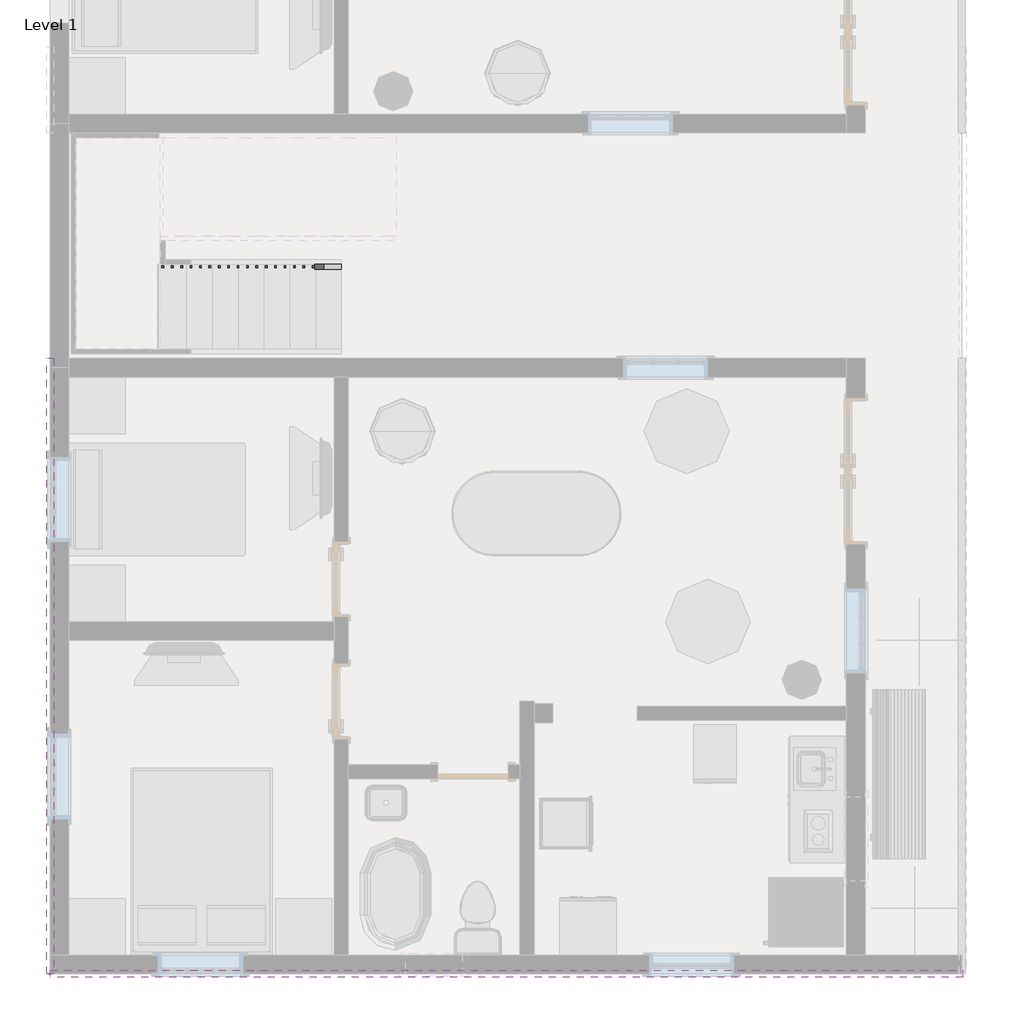
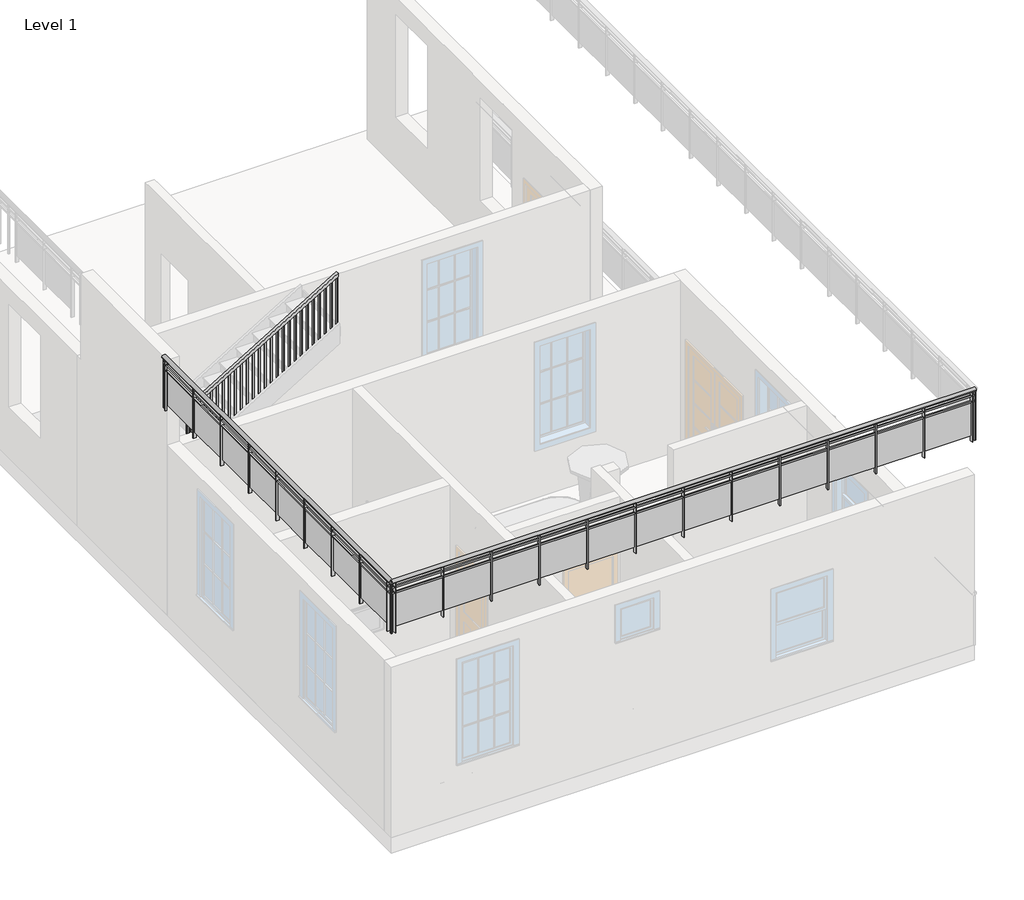
# One storey, part 2 of 4: 3 railings.
"""IFC4 building model written with IfcOpenShell, lengths in millimetres."""

from ifc_helpers import new_model, si_unit, point, frame, origin, place, context, project, spatial, polyline, ellipse_curve, trimmed, outline, extrude, faceted_brep, element, save
from ifc_brep_helpers import plane_surface, extruded_surface, advanced_brep

model = new_model("IFC4")

# Units and contexts
model_context = context("Model", 3, world=origin())
ifc_project = project(units=[si_unit("LENGTHUNIT", "METRE", prefix="MILLI")], contexts=[model_context])

# Site, building, storey
site = spatial("IfcSite", under=ifc_project)
building = spatial("IfcBuilding", under=site)
storey = spatial("IfcBuildingStorey", under=building, Name="Level 1", Elevation=0.0)

# Railings
placement = place(None, origin())
element("IfcRailing", 1, ObjectType="Glass Panel - Bottom Fill", at=placement, inside=storey, context=model_context, shape_type="SolidModel", body=[
    advanced_brep(
    [(-14570.2750862, -617.6379829, 4572.0), (-14570.2750862, -693.8379829, 4572.0), (-4702.3750862, -617.6379829, 4572.0), (-4702.3750862, -693.8379829, 4572.0)],
    [
        (0, 1, ellipse_curve(frame((-14570.2750862, -655.7379829, 4572.0), z_axis=(-1.0, 0.0, 0.0), x_axis=(0.0, -1.0, 0.0)), 38.1, 28.575)),
        (1, 0, ellipse_curve(frame((-14570.2750862, -655.7379829, 4572.0), z_axis=(-1.0, 0.0, 0.0), x_axis=(0.0, -1.0, 0.0)), 38.1, 28.575)),
        (2, 3, ellipse_curve(frame((-4702.3750862, -655.7379829, 4572.0), z_axis=(1.0, 0.0, 0.0), x_axis=(0.0, -1.0, 0.0)), 38.1, 28.575)),
        (3, 2, ellipse_curve(frame((-4702.3750862, -655.7379829, 4572.0), z_axis=(1.0, 0.0, 0.0), x_axis=(0.0, -1.0, 0.0)), 38.1, 28.575)),
        (0, 2),
        (3, 1),
    ],
    [
        plane_surface(frame((-14570.2750862, -655.7379829, 4572.0), z_axis=(-1.0, 0.0, 0.0), x_axis=(0.0, 1.0, 0.0))),
        plane_surface(frame((-4702.3750862, -655.7379829, 4572.0), z_axis=(1.0, 0.0, 0.0), x_axis=(0.0, 1.0, 0.0))),
        extruded_surface(trimmed(ellipse_curve(frame((-4702.3750862, -655.7379829, 4572.0), z_axis=(-1.0, 0.0, 0.0), x_axis=(0.0, -1.0, 0.0)), 38.1, 28.575), [point((-4702.3750862, -617.6379829, 4572.0))], [point((-4702.3750862, -693.8379829, 4572.0))], True, "CARTESIAN"), (-9867.9, 0.0, 0.0), 9867.9),
        extruded_surface(trimmed(ellipse_curve(frame((-4702.3750862, -655.7379829, 4572.0), z_axis=(-1.0, 0.0, 0.0), x_axis=(0.0, -1.0, 0.0)), 38.1, 28.575), [point((-4702.3750862, -693.8379829, 4572.0))], [point((-4702.3750862, -617.6379829, 4572.0))], True, "CARTESIAN"), (-9867.9, 0.0, 0.0), 9867.9),
    ],
    [
        (0, [[1, 2]]),
        (1, [[3, 4]]),
        (2, [[-1, 5, -4, 6]]),
        (3, [[-2, -6, -3, -5]]),
    ],
),
    extrude(outline(polyline([(-14570.2750862, -668.4379829), (-14570.2750862, -643.0379829), (-4702.3750862, -643.0379829), (-4702.3750862, -668.4379829), (-14570.2750862, -668.4379829)])), frame((0.0, 0.0, 4457.7), z_axis=(0.0, 0.0, 1.0), x_axis=(1.0, 0.0, 0.0)), (0.0, 0.0, 1.0), 25.4),
    extrude(outline(polyline([(-14570.2750862, -668.4379829), (-14570.2750862, -643.0379829), (-4702.3750862, -643.0379829), (-4702.3750862, -668.4379829), (-14570.2750862, -668.4379829)])), frame((0.0, 0.0, 4356.1), z_axis=(0.0, 0.0, 1.0), x_axis=(1.0, 0.0, 0.0)), (0.0, 0.0, 1.0), 25.4),
    extrude(outline(polyline([(-4765.8750862, -681.1379829), (-4765.8750862, -630.3379829), (-4753.1750862, -630.3379829), (-4753.1750862, -681.1379829), (-4765.8750862, -681.1379829)])), frame((0.0, 0.0, 3657.6), z_axis=(0.0, 0.0, 1.0), x_axis=(1.0, 0.0, 0.0)), (0.0, 0.0, 1.0), 885.6788223),
    extrude(outline(polyline([(-5572.3250862, -649.2028259), (-4759.5250862, -649.2028259), (-4759.5250862, -655.5528259), (-5572.3250862, -655.5528259), (-5572.3250862, -649.2028259)])), frame((0.0, 0.0, 3759.2), z_axis=(0.0, 0.0, 1.0), x_axis=(1.0, 0.0, 0.0)), (0.0, 0.0, 1.0), 596.9),
    extrude(outline(polyline([(-5578.6750862, -681.1379829), (-5578.6750862, -630.3379829), (-5565.9750862, -630.3379829), (-5565.9750862, -681.1379829), (-5578.6750862, -681.1379829)])), frame((0.0, 0.0, 3657.6), z_axis=(0.0, 0.0, 1.0), x_axis=(1.0, 0.0, 0.0)), (0.0, 0.0, 1.0), 885.6788223),
    extrude(outline(polyline([(-6385.1250862, -649.2028259), (-5572.3250862, -649.2028259), (-5572.3250862, -655.5528259), (-6385.1250862, -655.5528259), (-6385.1250862, -649.2028259)])), frame((0.0, 0.0, 3759.2), z_axis=(0.0, 0.0, 1.0), x_axis=(1.0, 0.0, 0.0)), (0.0, 0.0, 1.0), 596.9),
    extrude(outline(polyline([(-6391.4750862, -681.1379829), (-6391.4750862, -630.3379829), (-6378.7750862, -630.3379829), (-6378.7750862, -681.1379829), (-6391.4750862, -681.1379829)])), frame((0.0, 0.0, 3657.6), z_axis=(0.0, 0.0, 1.0), x_axis=(1.0, 0.0, 0.0)), (0.0, 0.0, 1.0), 885.6788223),
    extrude(outline(polyline([(-7197.9250862, -649.2028259), (-6385.1250862, -649.2028259), (-6385.1250862, -655.5528259), (-7197.9250862, -655.5528259), (-7197.9250862, -649.2028259)])), frame((0.0, 0.0, 3759.2), z_axis=(0.0, 0.0, 1.0), x_axis=(1.0, 0.0, 0.0)), (0.0, 0.0, 1.0), 596.9),
    extrude(outline(polyline([(-7204.2750862, -681.1379829), (-7204.2750862, -630.3379829), (-7191.5750862, -630.3379829), (-7191.5750862, -681.1379829), (-7204.2750862, -681.1379829)])), frame((0.0, 0.0, 3657.6), z_axis=(0.0, 0.0, 1.0), x_axis=(1.0, 0.0, 0.0)), (0.0, 0.0, 1.0), 885.6788223),
    extrude(outline(polyline([(-8010.7250862, -649.2028259), (-7197.9250862, -649.2028259), (-7197.9250862, -655.5528259), (-8010.7250862, -655.5528259), (-8010.7250862, -649.2028259)])), frame((0.0, 0.0, 3759.2), z_axis=(0.0, 0.0, 1.0), x_axis=(1.0, 0.0, 0.0)), (0.0, 0.0, 1.0), 596.9),
    extrude(outline(polyline([(-8017.0750862, -681.1379829), (-8017.0750862, -630.3379829), (-8004.3750862, -630.3379829), (-8004.3750862, -681.1379829), (-8017.0750862, -681.1379829)])), frame((0.0, 0.0, 3657.6), z_axis=(0.0, 0.0, 1.0), x_axis=(1.0, 0.0, 0.0)), (0.0, 0.0, 1.0), 885.6788223),
    extrude(outline(polyline([(-8823.5250862, -649.2028259), (-8010.7250862, -649.2028259), (-8010.7250862, -655.5528259), (-8823.5250862, -655.5528259), (-8823.5250862, -649.2028259)])), frame((0.0, 0.0, 3759.2), z_axis=(0.0, 0.0, 1.0), x_axis=(1.0, 0.0, 0.0)), (0.0, 0.0, 1.0), 596.9),
    extrude(outline(polyline([(-8829.8750862, -681.1379829), (-8829.8750862, -630.3379829), (-8817.1750862, -630.3379829), (-8817.1750862, -681.1379829), (-8829.8750862, -681.1379829)])), frame((0.0, 0.0, 3657.6), z_axis=(0.0, 0.0, 1.0), x_axis=(1.0, 0.0, 0.0)), (0.0, 0.0, 1.0), 885.6788223),
    extrude(outline(polyline([(-9636.3250862, -649.2028259), (-8823.5250862, -649.2028259), (-8823.5250862, -655.5528259), (-9636.3250862, -655.5528259), (-9636.3250862, -649.2028259)])), frame((0.0, 0.0, 3759.2), z_axis=(0.0, 0.0, 1.0), x_axis=(1.0, 0.0, 0.0)), (0.0, 0.0, 1.0), 596.9),
    extrude(outline(polyline([(-9642.6750862, -681.1379829), (-9642.6750862, -630.3379829), (-9629.9750862, -630.3379829), (-9629.9750862, -681.1379829), (-9642.6750862, -681.1379829)])), frame((0.0, 0.0, 3657.6), z_axis=(0.0, 0.0, 1.0), x_axis=(1.0, 0.0, 0.0)), (0.0, 0.0, 1.0), 885.6788223),
    extrude(outline(polyline([(-10449.1250862, -649.2028259), (-9636.3250862, -649.2028259), (-9636.3250862, -655.5528259), (-10449.1250862, -655.5528259), (-10449.1250862, -649.2028259)])), frame((0.0, 0.0, 3759.2), z_axis=(0.0, 0.0, 1.0), x_axis=(1.0, 0.0, 0.0)), (0.0, 0.0, 1.0), 596.9),
    extrude(outline(polyline([(-10455.4750862, -681.1379829), (-10455.4750862, -630.3379829), (-10442.7750862, -630.3379829), (-10442.7750862, -681.1379829), (-10455.4750862, -681.1379829)])), frame((0.0, 0.0, 3657.6), z_axis=(0.0, 0.0, 1.0), x_axis=(1.0, 0.0, 0.0)), (0.0, 0.0, 1.0), 885.6788223),
    extrude(outline(polyline([(-11261.9250862, -649.2028259), (-10449.1250862, -649.2028259), (-10449.1250862, -655.5528259), (-11261.9250862, -655.5528259), (-11261.9250862, -649.2028259)])), frame((0.0, 0.0, 3759.2), z_axis=(0.0, 0.0, 1.0), x_axis=(1.0, 0.0, 0.0)), (0.0, 0.0, 1.0), 596.9),
    extrude(outline(polyline([(-11268.2750862, -681.1379829), (-11268.2750862, -630.3379829), (-11255.5750862, -630.3379829), (-11255.5750862, -681.1379829), (-11268.2750862, -681.1379829)])), frame((0.0, 0.0, 3657.6), z_axis=(0.0, 0.0, 1.0), x_axis=(1.0, 0.0, 0.0)), (0.0, 0.0, 1.0), 885.6788223),
    extrude(outline(polyline([(-12074.7250862, -649.2028259), (-11261.9250862, -649.2028259), (-11261.9250862, -655.5528259), (-12074.7250862, -655.5528259), (-12074.7250862, -649.2028259)])), frame((0.0, 0.0, 3759.2), z_axis=(0.0, 0.0, 1.0), x_axis=(1.0, 0.0, 0.0)), (0.0, 0.0, 1.0), 596.9),
    extrude(outline(polyline([(-12081.0750862, -681.1379829), (-12081.0750862, -630.3379829), (-12068.3750862, -630.3379829), (-12068.3750862, -681.1379829), (-12081.0750862, -681.1379829)])), frame((0.0, 0.0, 3657.6), z_axis=(0.0, 0.0, 1.0), x_axis=(1.0, 0.0, 0.0)), (0.0, 0.0, 1.0), 885.6788223),
    extrude(outline(polyline([(-12887.5250862, -649.2028259), (-12074.7250862, -649.2028259), (-12074.7250862, -655.5528259), (-12887.5250862, -655.5528259), (-12887.5250862, -649.2028259)])), frame((0.0, 0.0, 3759.2), z_axis=(0.0, 0.0, 1.0), x_axis=(1.0, 0.0, 0.0)), (0.0, 0.0, 1.0), 596.9),
    extrude(outline(polyline([(-12893.8750862, -681.1379829), (-12893.8750862, -630.3379829), (-12881.1750862, -630.3379829), (-12881.1750862, -681.1379829), (-12893.8750862, -681.1379829)])), frame((0.0, 0.0, 3657.6), z_axis=(0.0, 0.0, 1.0), x_axis=(1.0, 0.0, 0.0)), (0.0, 0.0, 1.0), 885.6788223),
    extrude(outline(polyline([(-13700.3250862, -649.2028259), (-12887.5250862, -649.2028259), (-12887.5250862, -655.5528259), (-13700.3250862, -655.5528259), (-13700.3250862, -649.2028259)])), frame((0.0, 0.0, 3759.2), z_axis=(0.0, 0.0, 1.0), x_axis=(1.0, 0.0, 0.0)), (0.0, 0.0, 1.0), 596.9),
    extrude(outline(polyline([(-13706.6750862, -681.1379829), (-13706.6750862, -630.3379829), (-13693.9750862, -630.3379829), (-13693.9750862, -681.1379829), (-13706.6750862, -681.1379829)])), frame((0.0, 0.0, 3657.6), z_axis=(0.0, 0.0, 1.0), x_axis=(1.0, 0.0, 0.0)), (0.0, 0.0, 1.0), 885.6788223),
    extrude(outline(polyline([(-14513.1250862, -649.2028259), (-13700.3250862, -649.2028259), (-13700.3250862, -655.5528259), (-14513.1250862, -655.5528259), (-14513.1250862, -649.2028259)])), frame((0.0, 0.0, 3759.2), z_axis=(0.0, 0.0, 1.0), x_axis=(1.0, 0.0, 0.0)), (0.0, 0.0, 1.0), 596.9),
    extrude(outline(polyline([(-14519.4750862, -681.1379829), (-14519.4750862, -630.3379829), (-14506.7750862, -630.3379829), (-14506.7750862, -681.1379829), (-14519.4750862, -681.1379829)])), frame((0.0, 0.0, 3657.6), z_axis=(0.0, 0.0, 1.0), x_axis=(1.0, 0.0, 0.0)), (0.0, 0.0, 1.0), 885.6788223),
    extrude(outline(polyline([(-4715.0750862, -665.2629829), (-4715.0750862, -646.2129829), (-4696.0250862, -646.2129829), (-4696.0250862, -665.2629829), (-4715.0750862, -665.2629829)])), frame((0.0, 0.0, 3657.6), z_axis=(0.0, 0.0, 1.0), x_axis=(1.0, 0.0, 0.0)), (0.0, 0.0, 1.0), 885.6788223),
    extrude(outline(polyline([(-14576.6250862, -665.2629829), (-14576.6250862, -646.2129829), (-14557.5750862, -646.2129829), (-14557.5750862, -665.2629829), (-14576.6250862, -665.2629829)])), frame((0.0, 0.0, 3657.6), z_axis=(0.0, 0.0, 1.0), x_axis=(1.0, 0.0, 0.0)), (0.0, 0.0, 1.0), 885.6788223),
])
element("IfcRailing", 2, ObjectType="Glass Panel - Bottom Fill", at=placement, inside=storey, context=model_context, shape_type="SolidModel", body=[
    advanced_brep(
    [(-14532.1750862, 5999.0620171, 4572.0), (-14608.3750862, 5999.0620171, 4572.0), (-14532.1750862, -655.7379829, 4572.0), (-14608.3750862, -655.7379829, 4572.0)],
    [
        (0, 1, ellipse_curve(frame((-14570.2750862, 5999.0620171, 4572.0), z_axis=(0.0, 1.0, 0.0), x_axis=(-1.0, 0.0, 0.0)), 38.1, 28.575)),
        (1, 0, ellipse_curve(frame((-14570.2750862, 5999.0620171, 4572.0), z_axis=(0.0, 1.0, 0.0), x_axis=(-1.0, 0.0, 0.0)), 38.1, 28.575)),
        (2, 3, ellipse_curve(frame((-14570.2750862, -655.7379829, 4572.0), z_axis=(0.0, -1.0, 0.0), x_axis=(-1.0, 0.0, 0.0)), 38.1, 28.575)),
        (3, 2, ellipse_curve(frame((-14570.2750862, -655.7379829, 4572.0), z_axis=(0.0, -1.0, 0.0), x_axis=(-1.0, 0.0, 0.0)), 38.1, 28.575)),
        (0, 2),
        (3, 1),
    ],
    [
        plane_surface(frame((-14570.2750862, 5999.0620171, 4572.0), z_axis=(0.0, 1.0, 0.0), x_axis=(0.0, 0.0, -1.0))),
        plane_surface(frame((-14570.2750862, -655.7379829, 4572.0), z_axis=(0.0, -1.0, 0.0), x_axis=(0.0, 0.0, -1.0))),
        extruded_surface(trimmed(ellipse_curve(frame((-14570.2750862, -655.7379829, 4572.0), z_axis=(0.0, 1.0, 0.0), x_axis=(-1.0, 0.0, 0.0)), 38.1, 28.575), [point((-14532.1750862, -655.7379829, 4572.0))], [point((-14608.3750862, -655.7379829, 4572.0))], True, "CARTESIAN"), (0.0, 6654.8, 0.0), 6654.8),
        extruded_surface(trimmed(ellipse_curve(frame((-14570.2750862, -655.7379829, 4572.0), z_axis=(0.0, 1.0, 0.0), x_axis=(-1.0, 0.0, 0.0)), 38.1, 28.575), [point((-14608.3750862, -655.7379829, 4572.0))], [point((-14532.1750862, -655.7379829, 4572.0))], True, "CARTESIAN"), (0.0, 6654.8, 0.0), 6654.8),
    ],
    [
        (0, [[1, 2]]),
        (1, [[3, 4]]),
        (2, [[-1, 5, -4, 6]]),
        (3, [[-2, -6, -3, -5]]),
    ],
),
    extrude(outline(polyline([(-14582.9750862, 5999.0620171), (-14557.5750862, 5999.0620171), (-14557.5750862, -655.7379829), (-14582.9750862, -655.7379829), (-14582.9750862, 5999.0620171)])), frame((0.0, 0.0, 4457.7), z_axis=(0.0, 0.0, 1.0), x_axis=(1.0, 0.0, 0.0)), (0.0, 0.0, 1.0), 25.4),
    extrude(outline(polyline([(-14582.9750862, 5999.0620171), (-14557.5750862, 5999.0620171), (-14557.5750862, -655.7379829), (-14582.9750862, -655.7379829), (-14582.9750862, 5999.0620171)])), frame((0.0, 0.0, 4356.1), z_axis=(0.0, 0.0, 1.0), x_axis=(1.0, 0.0, 0.0)), (0.0, 0.0, 1.0), 25.4),
    extrude(outline(polyline([(-14595.6750862, -573.1879829), (-14544.8750862, -573.1879829), (-14544.8750862, -585.8879829), (-14595.6750862, -585.8879829), (-14595.6750862, -573.1879829)])), frame((0.0, 0.0, 3657.6), z_axis=(0.0, 0.0, 1.0), x_axis=(1.0, 0.0, 0.0)), (0.0, 0.0, 1.0), 885.6788223),
    extrude(outline(polyline([(-14563.7399292, 233.2620171), (-14563.7399292, -579.5379829), (-14570.0899292, -579.5379829), (-14570.0899292, 233.2620171), (-14563.7399292, 233.2620171)])), frame((0.0, 0.0, 3759.2), z_axis=(0.0, 0.0, 1.0), x_axis=(1.0, 0.0, 0.0)), (0.0, 0.0, 1.0), 596.9),
    extrude(outline(polyline([(-14595.6750862, 239.6120171), (-14544.8750862, 239.6120171), (-14544.8750862, 226.9120171), (-14595.6750862, 226.9120171), (-14595.6750862, 239.6120171)])), frame((0.0, 0.0, 3657.6), z_axis=(0.0, 0.0, 1.0), x_axis=(1.0, 0.0, 0.0)), (0.0, 0.0, 1.0), 885.6788223),
    extrude(outline(polyline([(-14563.7399292, 1046.0620171), (-14563.7399292, 233.2620171), (-14570.0899292, 233.2620171), (-14570.0899292, 1046.0620171), (-14563.7399292, 1046.0620171)])), frame((0.0, 0.0, 3759.2), z_axis=(0.0, 0.0, 1.0), x_axis=(1.0, 0.0, 0.0)), (0.0, 0.0, 1.0), 596.9),
    extrude(outline(polyline([(-14595.6750862, 1052.4120171), (-14544.8750862, 1052.4120171), (-14544.8750862, 1039.7120171), (-14595.6750862, 1039.7120171), (-14595.6750862, 1052.4120171)])), frame((0.0, 0.0, 3657.6), z_axis=(0.0, 0.0, 1.0), x_axis=(1.0, 0.0, 0.0)), (0.0, 0.0, 1.0), 885.6788223),
    extrude(outline(polyline([(-14563.7399292, 1858.8620171), (-14563.7399292, 1046.0620171), (-14570.0899292, 1046.0620171), (-14570.0899292, 1858.8620171), (-14563.7399292, 1858.8620171)])), frame((0.0, 0.0, 3759.2), z_axis=(0.0, 0.0, 1.0), x_axis=(1.0, 0.0, 0.0)), (0.0, 0.0, 1.0), 596.9),
    extrude(outline(polyline([(-14595.6750862, 1865.2120171), (-14544.8750862, 1865.2120171), (-14544.8750862, 1852.5120171), (-14595.6750862, 1852.5120171), (-14595.6750862, 1865.2120171)])), frame((0.0, 0.0, 3657.6), z_axis=(0.0, 0.0, 1.0), x_axis=(1.0, 0.0, 0.0)), (0.0, 0.0, 1.0), 885.6788223),
    extrude(outline(polyline([(-14563.7399292, 2671.6620171), (-14563.7399292, 1858.8620171), (-14570.0899292, 1858.8620171), (-14570.0899292, 2671.6620171), (-14563.7399292, 2671.6620171)])), frame((0.0, 0.0, 3759.2), z_axis=(0.0, 0.0, 1.0), x_axis=(1.0, 0.0, 0.0)), (0.0, 0.0, 1.0), 596.9),
    extrude(outline(polyline([(-14595.6750862, 2678.0120171), (-14544.8750862, 2678.0120171), (-14544.8750862, 2665.3120171), (-14595.6750862, 2665.3120171), (-14595.6750862, 2678.0120171)])), frame((0.0, 0.0, 3657.6), z_axis=(0.0, 0.0, 1.0), x_axis=(1.0, 0.0, 0.0)), (0.0, 0.0, 1.0), 885.6788223),
    extrude(outline(polyline([(-14563.7399292, 3484.4620171), (-14563.7399292, 2671.6620171), (-14570.0899292, 2671.6620171), (-14570.0899292, 3484.4620171), (-14563.7399292, 3484.4620171)])), frame((0.0, 0.0, 3759.2), z_axis=(0.0, 0.0, 1.0), x_axis=(1.0, 0.0, 0.0)), (0.0, 0.0, 1.0), 596.9),
    extrude(outline(polyline([(-14595.6750862, 3490.8120171), (-14544.8750862, 3490.8120171), (-14544.8750862, 3478.1120171), (-14595.6750862, 3478.1120171), (-14595.6750862, 3490.8120171)])), frame((0.0, 0.0, 3657.6), z_axis=(0.0, 0.0, 1.0), x_axis=(1.0, 0.0, 0.0)), (0.0, 0.0, 1.0), 885.6788223),
    extrude(outline(polyline([(-14563.7399292, 4297.2620171), (-14563.7399292, 3484.4620171), (-14570.0899292, 3484.4620171), (-14570.0899292, 4297.2620171), (-14563.7399292, 4297.2620171)])), frame((0.0, 0.0, 3759.2), z_axis=(0.0, 0.0, 1.0), x_axis=(1.0, 0.0, 0.0)), (0.0, 0.0, 1.0), 596.9),
    extrude(outline(polyline([(-14595.6750862, 4303.6120171), (-14544.8750862, 4303.6120171), (-14544.8750862, 4290.9120171), (-14595.6750862, 4290.9120171), (-14595.6750862, 4303.6120171)])), frame((0.0, 0.0, 3657.6), z_axis=(0.0, 0.0, 1.0), x_axis=(1.0, 0.0, 0.0)), (0.0, 0.0, 1.0), 885.6788223),
    extrude(outline(polyline([(-14563.7399292, 5110.0620171), (-14563.7399292, 4297.2620171), (-14570.0899292, 4297.2620171), (-14570.0899292, 5110.0620171), (-14563.7399292, 5110.0620171)])), frame((0.0, 0.0, 3759.2), z_axis=(0.0, 0.0, 1.0), x_axis=(1.0, 0.0, 0.0)), (0.0, 0.0, 1.0), 596.9),
    extrude(outline(polyline([(-14595.6750862, 5116.4120171), (-14544.8750862, 5116.4120171), (-14544.8750862, 5103.7120171), (-14595.6750862, 5103.7120171), (-14595.6750862, 5116.4120171)])), frame((0.0, 0.0, 3657.6), z_axis=(0.0, 0.0, 1.0), x_axis=(1.0, 0.0, 0.0)), (0.0, 0.0, 1.0), 885.6788223),
    extrude(outline(polyline([(-14563.7399292, 5922.8620171), (-14563.7399292, 5110.0620171), (-14570.0899292, 5110.0620171), (-14570.0899292, 5922.8620171), (-14563.7399292, 5922.8620171)])), frame((0.0, 0.0, 3759.2), z_axis=(0.0, 0.0, 1.0), x_axis=(1.0, 0.0, 0.0)), (0.0, 0.0, 1.0), 596.9),
    extrude(outline(polyline([(-14595.6750862, 5929.2120171), (-14544.8750862, 5929.2120171), (-14544.8750862, 5916.5120171), (-14595.6750862, 5916.5120171), (-14595.6750862, 5929.2120171)])), frame((0.0, 0.0, 3657.6), z_axis=(0.0, 0.0, 1.0), x_axis=(1.0, 0.0, 0.0)), (0.0, 0.0, 1.0), 885.6788223),
    extrude(outline(polyline([(-14579.8000862, -643.0379829), (-14560.7500862, -643.0379829), (-14560.7500862, -662.0879829), (-14579.8000862, -662.0879829), (-14579.8000862, -643.0379829)])), frame((0.0, 0.0, 3657.6), z_axis=(0.0, 0.0, 1.0), x_axis=(1.0, 0.0, 0.0)), (0.0, 0.0, 1.0), 885.6788223),
    extrude(outline(polyline([(-14579.8000862, 6005.4120171), (-14560.7500862, 6005.4120171), (-14560.7500862, 5986.3620171), (-14579.8000862, 5986.3620171), (-14579.8000862, 6005.4120171)])), frame((0.0, 0.0, 3657.6), z_axis=(0.0, 0.0, 1.0), x_axis=(1.0, 0.0, 0.0)), (0.0, 0.0, 1.0), 885.6788223),
])
element("IfcRailing", 3, ObjectType="Handrail - Rectangular", at=placement, inside=storey, context=model_context, shape_type="SolidModel", body=[
    faceted_brep([(-11420.6750862, 6964.2620171, 1083.7333333), (-11420.6750862, 6964.2620171, 1024.3318731), (-11420.6750862, 7015.0620171, 1024.3318731), (-11420.6750862, 7015.0620171, 1083.7333333), (-13300.2750862, 6964.2620171, 2222.8848485), (-13351.0750862, 6964.2620171, 2194.271267), (-13351.0750862, 7015.0620171, 2194.271267), (-13300.2750862, 7015.0620171, 2222.8848485), (-13300.2750862, 6964.2620171, 2269.0666667), (-13351.0750862, 6964.2620171, 2218.2666667), (-13351.0750862, 7015.0620171, 2218.2666667), (-13300.2750862, 7015.0620171, 2269.0666667), (-13427.2750862, 6964.2620171, 2269.0666667), (-13427.2750862, 6964.2620171, 2218.2666667), (-13376.4750862, 7015.0620171, 2218.2666667), (-13376.4750862, 7015.0620171, 2269.0666667), (-13427.2750862, 7091.2620171, 2269.0666667), (-13427.2750862, 7091.2620171, 2218.2666667), (-13376.4750862, 7091.2620171, 2218.2666667), (-13376.4750862, 7091.2620171, 2269.0666667), (-13427.2750862, 7243.6620171, 2269.0666667), (-13427.2750862, 7294.4620171, 2218.2666667), (-13376.4750862, 7294.4620171, 2218.2666667), (-13376.4750862, 7243.6620171, 2269.0666667), (-13427.2750862, 7243.6620171, 2484.5818182), (-13427.2750862, 7294.4620171, 2433.7818182), (-13376.4750862, 7294.4620171, 2433.7818182), (-13376.4750862, 7243.6620171, 2484.5818182), (-13427.2750862, 7370.6620171, 2484.5818182), (-13427.2750862, 7370.6620171, 2433.7818182), (-13376.4750862, 7319.8620171, 2433.7818182), (-13376.4750862, 7319.8620171, 2484.5818182), (-13300.2750862, 7370.6620171, 2484.5818182), (-13286.0826767, 7370.6620171, 2433.7818182), (-13286.0826767, 7319.8620171, 2433.7818182), (-13300.2750862, 7319.8620171, 2484.5818182), (-10861.8750862, 7370.6620171, 3962.4), (-10861.8750862, 7319.8620171, 3962.4), (-10861.8750862, 7319.8620171, 3902.9985397), (-10861.8750862, 7370.6620171, 3902.9985397)], [[[0, 1, 2, 3]], [[1, 0, 4, 5]], [[2, 1, 5, 6]], [[3, 2, 6, 7]], [[0, 3, 7, 4]], [[5, 4, 8, 9]], [[6, 5, 9, 10]], [[7, 6, 10, 11]], [[4, 7, 11, 8]], [[9, 8, 12, 13]], [[10, 9, 13, 14]], [[11, 10, 14, 15]], [[8, 11, 15, 12]], [[13, 12, 16, 17]], [[14, 13, 17, 18]], [[15, 14, 18, 19]], [[12, 15, 19, 16]], [[17, 16, 20, 21]], [[18, 17, 21, 22]], [[19, 18, 22, 23]], [[16, 19, 23, 20]], [[21, 20, 24, 25]], [[22, 21, 25, 26]], [[23, 22, 26, 27]], [[20, 23, 27, 24]], [[25, 24, 28, 29]], [[26, 25, 29, 30]], [[27, 26, 30, 31]], [[24, 27, 31, 28]], [[29, 28, 32, 33]], [[30, 29, 33, 34]], [[31, 30, 34, 35]], [[28, 31, 35, 32]], [[36, 37, 38, 39]], [[33, 32, 36, 39]], [[34, 33, 39, 38]], [[35, 34, 38, 37]], [[32, 35, 37, 36]]]),
    extrude(outline(polyline([(3847.1955094, -10953.9500862), (3835.6500549, -10973.0000862), (2878.6666667, -10973.0000862), (2878.6666667, -10953.9500862), (3847.1955094, -10953.9500862)])), frame((0.0, 7335.7370171, 0.0), z_axis=(0.0, 1.0, 0.0), x_axis=(0.0, 0.0, 1.0)), (0.0, 0.0, 1.0), 19.05),
    extrude(outline(polyline([(3785.6197519, -11055.5500862), (3774.0742973, -11074.6000862), (2878.6666667, -11074.6000862), (2878.6666667, -11055.5500862), (3785.6197519, -11055.5500862)])), frame((0.0, 7335.7370171, 0.0), z_axis=(0.0, 1.0, 0.0), x_axis=(0.0, 0.0, 1.0)), (0.0, 0.0, 1.0), 19.05),
    extrude(outline(polyline([(3724.0439943, -11157.1500862), (3712.4985397, -11176.2000862), (2709.3333333, -11176.2000862), (2709.3333333, -11157.1500862), (3724.0439943, -11157.1500862)])), frame((0.0, 7335.7370171, 0.0), z_axis=(0.0, 1.0, 0.0), x_axis=(0.0, 0.0, 1.0)), (0.0, 0.0, 1.0), 19.05),
    extrude(outline(polyline([(3662.4682367, -11258.7500862), (3650.9227822, -11277.8000862), (2709.3333333, -11277.8000862), (2709.3333333, -11258.7500862), (3662.4682367, -11258.7500862)])), frame((0.0, 7335.7370171, 0.0), z_axis=(0.0, 1.0, 0.0), x_axis=(0.0, 0.0, 1.0)), (0.0, 0.0, 1.0), 19.05),
    extrude(outline(polyline([(3600.8924791, -11360.3500862), (3589.3470246, -11379.4000862), (2709.3333333, -11379.4000862), (2709.3333333, -11360.3500862), (3600.8924791, -11360.3500862)])), frame((0.0, 7335.7370171, 0.0), z_axis=(0.0, 1.0, 0.0), x_axis=(0.0, 0.0, 1.0)), (0.0, 0.0, 1.0), 19.05),
    extrude(outline(polyline([(3539.3167216, -11461.9500862), (3527.771267, -11481.0000862), (2540.0, -11481.0000862), (2540.0, -11461.9500862), (3539.3167216, -11461.9500862)])), frame((0.0, 7335.7370171, 0.0), z_axis=(0.0, 1.0, 0.0), x_axis=(0.0, 0.0, 1.0)), (0.0, 0.0, 1.0), 19.05),
    extrude(outline(polyline([(3477.740964, -11563.5500862), (3466.1955094, -11582.6000862), (2540.0, -11582.6000862), (2540.0, -11563.5500862), (3477.740964, -11563.5500862)])), frame((0.0, 7335.7370171, 0.0), z_axis=(0.0, 1.0, 0.0), x_axis=(0.0, 0.0, 1.0)), (0.0, 0.0, 1.0), 19.05),
    extrude(outline(polyline([(3416.1652064, -11665.1500862), (3404.6197519, -11684.2000862), (2540.0, -11684.2000862), (2540.0, -11665.1500862), (3416.1652064, -11665.1500862)])), frame((0.0, 7335.7370171, 0.0), z_axis=(0.0, 1.0, 0.0), x_axis=(0.0, 0.0, 1.0)), (0.0, 0.0, 1.0), 19.05),
    extrude(outline(polyline([(3354.5894488, -11766.7500862), (3343.0439943, -11785.8000862), (2370.6666667, -11785.8000862), (2370.6666667, -11766.7500862), (3354.5894488, -11766.7500862)])), frame((0.0, 7335.7370171, 0.0), z_axis=(0.0, 1.0, 0.0), x_axis=(0.0, 0.0, 1.0)), (0.0, 0.0, 1.0), 19.05),
    extrude(outline(polyline([(3293.0136913, -11868.3500862), (3281.4682367, -11887.4000862), (2370.6666667, -11887.4000862), (2370.6666667, -11868.3500862), (3293.0136913, -11868.3500862)])), frame((0.0, 7335.7370171, 0.0), z_axis=(0.0, 1.0, 0.0), x_axis=(0.0, 0.0, 1.0)), (0.0, 0.0, 1.0), 19.05),
    extrude(outline(polyline([(3231.4379337, -11969.9500862), (3219.8924791, -11989.0000862), (2370.6666667, -11989.0000862), (2370.6666667, -11969.9500862), (3231.4379337, -11969.9500862)])), frame((0.0, 7335.7370171, 0.0), z_axis=(0.0, 1.0, 0.0), x_axis=(0.0, 0.0, 1.0)), (0.0, 0.0, 1.0), 19.05),
    extrude(outline(polyline([(3169.8621761, -12071.5500862), (3158.3167216, -12090.6000862), (2201.3333333, -12090.6000862), (2201.3333333, -12071.5500862), (3169.8621761, -12071.5500862)])), frame((0.0, 7335.7370171, 0.0), z_axis=(0.0, 1.0, 0.0), x_axis=(0.0, 0.0, 1.0)), (0.0, 0.0, 1.0), 19.05),
    extrude(outline(polyline([(3108.2864185, -12173.1500862), (3096.740964, -12192.2000862), (2201.3333333, -12192.2000862), (2201.3333333, -12173.1500862), (3108.2864185, -12173.1500862)])), frame((0.0, 7335.7370171, 0.0), z_axis=(0.0, 1.0, 0.0), x_axis=(0.0, 0.0, 1.0)), (0.0, 0.0, 1.0), 19.05),
    extrude(outline(polyline([(3046.710661, -12274.7500862), (3035.1652064, -12293.8000862), (2032.0, -12293.8000862), (2032.0, -12274.7500862), (3046.710661, -12274.7500862)])), frame((0.0, 7335.7370171, 0.0), z_axis=(0.0, 1.0, 0.0), x_axis=(0.0, 0.0, 1.0)), (0.0, 0.0, 1.0), 19.05),
    extrude(outline(polyline([(2985.1349034, -12376.3500862), (2973.5894488, -12395.4000862), (2032.0, -12395.4000862), (2032.0, -12376.3500862), (2985.1349034, -12376.3500862)])), frame((0.0, 7335.7370171, 0.0), z_axis=(0.0, 1.0, 0.0), x_axis=(0.0, 0.0, 1.0)), (0.0, 0.0, 1.0), 19.05),
    extrude(outline(polyline([(2923.5591458, -12477.9500862), (2912.0136913, -12497.0000862), (2032.0, -12497.0000862), (2032.0, -12477.9500862), (2923.5591458, -12477.9500862)])), frame((0.0, 7335.7370171, 0.0), z_axis=(0.0, 1.0, 0.0), x_axis=(0.0, 0.0, 1.0)), (0.0, 0.0, 1.0), 19.05),
    extrude(outline(polyline([(2861.9833882, -12579.5500862), (2850.4379337, -12598.6000862), (1862.6666667, -12598.6000862), (1862.6666667, -12579.5500862), (2861.9833882, -12579.5500862)])), frame((0.0, 7335.7370171, 0.0), z_axis=(0.0, 1.0, 0.0), x_axis=(0.0, 0.0, 1.0)), (0.0, 0.0, 1.0), 19.05),
    extrude(outline(polyline([(2800.4076307, -12681.1500862), (2788.8621761, -12700.2000862), (1862.6666667, -12700.2000862), (1862.6666667, -12681.1500862), (2800.4076307, -12681.1500862)])), frame((0.0, 7335.7370171, 0.0), z_axis=(0.0, 1.0, 0.0), x_axis=(0.0, 0.0, 1.0)), (0.0, 0.0, 1.0), 19.05),
    extrude(outline(polyline([(2738.8318731, -12782.7500862), (2727.2864185, -12801.8000862), (1862.6666667, -12801.8000862), (1862.6666667, -12782.7500862), (2738.8318731, -12782.7500862)])), frame((0.0, 7335.7370171, 0.0), z_axis=(0.0, 1.0, 0.0), x_axis=(0.0, 0.0, 1.0)), (0.0, 0.0, 1.0), 19.05),
    extrude(outline(polyline([(2677.2561155, -12884.3500862), (2665.710661, -12903.4000862), (1693.3333333, -12903.4000862), (1693.3333333, -12884.3500862), (2677.2561155, -12884.3500862)])), frame((0.0, 7335.7370171, 0.0), z_axis=(0.0, 1.0, 0.0), x_axis=(0.0, 0.0, 1.0)), (0.0, 0.0, 1.0), 19.05),
    extrude(outline(polyline([(2615.6803579, -12985.9500862), (2604.1349034, -13005.0000862), (1693.3333333, -13005.0000862), (1693.3333333, -12985.9500862), (2615.6803579, -12985.9500862)])), frame((0.0, 7335.7370171, 0.0), z_axis=(0.0, 1.0, 0.0), x_axis=(0.0, 0.0, 1.0)), (0.0, 0.0, 1.0), 19.05),
    extrude(outline(polyline([(2554.1046004, -13087.5500862), (2542.5591458, -13106.6000862), (1693.3333333, -13106.6000862), (1693.3333333, -13087.5500862), (2554.1046004, -13087.5500862)])), frame((0.0, 7335.7370171, 0.0), z_axis=(0.0, 1.0, 0.0), x_axis=(0.0, 0.0, 1.0)), (0.0, 0.0, 1.0), 19.05),
    extrude(outline(polyline([(2492.5288428, -13189.1500862), (2480.9833882, -13208.2000862), (1524.0, -13208.2000862), (1524.0, -13189.1500862), (2492.5288428, -13189.1500862)])), frame((0.0, 7335.7370171, 0.0), z_axis=(0.0, 1.0, 0.0), x_axis=(0.0, 0.0, 1.0)), (0.0, 0.0, 1.0), 19.05),
    extrude(outline(polyline([(-13309.8000862, 7335.7370171), (-13309.8000862, 7354.7870171), (-13290.7500862, 7354.7870171), (-13290.7500862, 7335.7370171), (-13309.8000862, 7335.7370171)])), frame((0.0, 0.0, 1524.0), z_axis=(0.0, 0.0, 1.0), x_axis=(1.0, 0.0, 0.0)), (0.0, 0.0, 1.0), 909.7818182),
    extrude(outline(polyline([(-13392.3500862, 7284.9370171), (-13411.4000862, 7284.9370171), (-13411.4000862, 7303.9870171), (-13392.3500862, 7303.9870171), (-13392.3500862, 7284.9370171)])), frame((0.0, 0.0, 1354.6666667), z_axis=(0.0, 0.0, 1.0), x_axis=(1.0, 0.0, 0.0)), (0.0, 0.0, 1.0), 863.6),
    extrude(outline(polyline([(-13392.3500862, 7183.3370171), (-13411.4000862, 7183.3370171), (-13411.4000862, 7202.3870171), (-13392.3500862, 7202.3870171), (-13392.3500862, 7183.3370171)])), frame((0.0, 0.0, 1354.6666667), z_axis=(0.0, 0.0, 1.0), x_axis=(1.0, 0.0, 0.0)), (0.0, 0.0, 1.0), 863.6),
    extrude(outline(polyline([(-13392.3500862, 7081.7370171), (-13411.4000862, 7081.7370171), (-13411.4000862, 7100.7870171), (-13392.3500862, 7100.7870171), (-13392.3500862, 7081.7370171)])), frame((0.0, 0.0, 1354.6666667), z_axis=(0.0, 0.0, 1.0), x_axis=(1.0, 0.0, 0.0)), (0.0, 0.0, 1.0), 863.6),
    extrude(outline(polyline([(2188.4985397, -13341.5500862), (2200.0439943, -13360.6000862), (1185.3333333, -13360.6000862), (1185.3333333, -13341.5500862), (2188.4985397, -13341.5500862)])), frame((0.0, 6980.1370171, 0.0), z_axis=(0.0, 1.0, 0.0), x_axis=(0.0, 0.0, 1.0)), (0.0, 0.0, 1.0), 19.05),
    extrude(outline(polyline([(2126.9227822, -13239.9500862), (2138.4682367, -13259.0000862), (1185.3333333, -13259.0000862), (1185.3333333, -13239.9500862), (2126.9227822, -13239.9500862)])), frame((0.0, 6980.1370171, 0.0), z_axis=(0.0, 1.0, 0.0), x_axis=(0.0, 0.0, 1.0)), (0.0, 0.0, 1.0), 19.05),
    extrude(outline(polyline([(2065.3470246, -13138.3500862), (2076.8924791, -13157.4000862), (1185.3333333, -13157.4000862), (1185.3333333, -13138.3500862), (2065.3470246, -13138.3500862)])), frame((0.0, 6980.1370171, 0.0), z_axis=(0.0, 1.0, 0.0), x_axis=(0.0, 0.0, 1.0)), (0.0, 0.0, 1.0), 19.05),
    extrude(outline(polyline([(2003.771267, -13036.7500862), (2015.3167216, -13055.8000862), (1016.0, -13055.8000862), (1016.0, -13036.7500862), (2003.771267, -13036.7500862)])), frame((0.0, 6980.1370171, 0.0), z_axis=(0.0, 1.0, 0.0), x_axis=(0.0, 0.0, 1.0)), (0.0, 0.0, 1.0), 19.05),
    extrude(outline(polyline([(1942.1955094, -12935.1500862), (1953.740964, -12954.2000862), (1016.0, -12954.2000862), (1016.0, -12935.1500862), (1942.1955094, -12935.1500862)])), frame((0.0, 6980.1370171, 0.0), z_axis=(0.0, 1.0, 0.0), x_axis=(0.0, 0.0, 1.0)), (0.0, 0.0, 1.0), 19.05),
    extrude(outline(polyline([(1880.6197519, -12833.5500862), (1892.1652064, -12852.6000862), (1016.0, -12852.6000862), (1016.0, -12833.5500862), (1880.6197519, -12833.5500862)])), frame((0.0, 6980.1370171, 0.0), z_axis=(0.0, 1.0, 0.0), x_axis=(0.0, 0.0, 1.0)), (0.0, 0.0, 1.0), 19.05),
    extrude(outline(polyline([(1819.0439943, -12731.9500862), (1830.5894488, -12751.0000862), (846.6666667, -12751.0000862), (846.6666667, -12731.9500862), (1819.0439943, -12731.9500862)])), frame((0.0, 6980.1370171, 0.0), z_axis=(0.0, 1.0, 0.0), x_axis=(0.0, 0.0, 1.0)), (0.0, 0.0, 1.0), 19.05),
    extrude(outline(polyline([(1757.4682367, -12630.3500862), (1769.0136913, -12649.4000862), (846.6666667, -12649.4000862), (846.6666667, -12630.3500862), (1757.4682367, -12630.3500862)])), frame((0.0, 6980.1370171, 0.0), z_axis=(0.0, 1.0, 0.0), x_axis=(0.0, 0.0, 1.0)), (0.0, 0.0, 1.0), 19.05),
    extrude(outline(polyline([(1695.8924791, -12528.7500862), (1707.4379337, -12547.8000862), (846.6666667, -12547.8000862), (846.6666667, -12528.7500862), (1695.8924791, -12528.7500862)])), frame((0.0, 6980.1370171, 0.0), z_axis=(0.0, 1.0, 0.0), x_axis=(0.0, 0.0, 1.0)), (0.0, 0.0, 1.0), 19.05),
    extrude(outline(polyline([(1634.3167216, -12427.1500862), (1645.8621761, -12446.2000862), (677.3333333, -12446.2000862), (677.3333333, -12427.1500862), (1634.3167216, -12427.1500862)])), frame((0.0, 6980.1370171, 0.0), z_axis=(0.0, 1.0, 0.0), x_axis=(0.0, 0.0, 1.0)), (0.0, 0.0, 1.0), 19.05),
    extrude(outline(polyline([(1572.740964, -12325.5500862), (1584.2864185, -12344.6000862), (677.3333333, -12344.6000862), (677.3333333, -12325.5500862), (1572.740964, -12325.5500862)])), frame((0.0, 6980.1370171, 0.0), z_axis=(0.0, 1.0, 0.0), x_axis=(0.0, 0.0, 1.0)), (0.0, 0.0, 1.0), 19.05),
    extrude(outline(polyline([(1511.1652064, -12223.9500862), (1522.710661, -12243.0000862), (508.0, -12243.0000862), (508.0, -12223.9500862), (1511.1652064, -12223.9500862)])), frame((0.0, 6980.1370171, 0.0), z_axis=(0.0, 1.0, 0.0), x_axis=(0.0, 0.0, 1.0)), (0.0, 0.0, 1.0), 19.05),
    extrude(outline(polyline([(1449.5894488, -12122.3500862), (1461.1349034, -12141.4000862), (508.0, -12141.4000862), (508.0, -12122.3500862), (1449.5894488, -12122.3500862)])), frame((0.0, 6980.1370171, 0.0), z_axis=(0.0, 1.0, 0.0), x_axis=(0.0, 0.0, 1.0)), (0.0, 0.0, 1.0), 19.05),
    extrude(outline(polyline([(1388.0136913, -12020.7500862), (1399.5591458, -12039.8000862), (508.0, -12039.8000862), (508.0, -12020.7500862), (1388.0136913, -12020.7500862)])), frame((0.0, 6980.1370171, 0.0), z_axis=(0.0, 1.0, 0.0), x_axis=(0.0, 0.0, 1.0)), (0.0, 0.0, 1.0), 19.05),
    extrude(outline(polyline([(1326.4379337, -11919.1500862), (1337.9833882, -11938.2000862), (338.6666667, -11938.2000862), (338.6666667, -11919.1500862), (1326.4379337, -11919.1500862)])), frame((0.0, 6980.1370171, 0.0), z_axis=(0.0, 1.0, 0.0), x_axis=(0.0, 0.0, 1.0)), (0.0, 0.0, 1.0), 19.05),
    extrude(outline(polyline([(1264.8621761, -11817.5500862), (1276.4076307, -11836.6000862), (338.6666667, -11836.6000862), (338.6666667, -11817.5500862), (1264.8621761, -11817.5500862)])), frame((0.0, 6980.1370171, 0.0), z_axis=(0.0, 1.0, 0.0), x_axis=(0.0, 0.0, 1.0)), (0.0, 0.0, 1.0), 19.05),
    extrude(outline(polyline([(1203.2864185, -11715.9500862), (1214.8318731, -11735.0000862), (338.6666667, -11735.0000862), (338.6666667, -11715.9500862), (1203.2864185, -11715.9500862)])), frame((0.0, 6980.1370171, 0.0), z_axis=(0.0, 1.0, 0.0), x_axis=(0.0, 0.0, 1.0)), (0.0, 0.0, 1.0), 19.05),
    extrude(outline(polyline([(1141.710661, -11614.3500862), (1153.2561155, -11633.4000862), (169.3333333, -11633.4000862), (169.3333333, -11614.3500862), (1141.710661, -11614.3500862)])), frame((0.0, 6980.1370171, 0.0), z_axis=(0.0, 1.0, 0.0), x_axis=(0.0, 0.0, 1.0)), (0.0, 0.0, 1.0), 19.05),
    extrude(outline(polyline([(1080.1349034, -11512.7500862), (1091.6803579, -11531.8000862), (169.3333333, -11531.8000862), (169.3333333, -11512.7500862), (1080.1349034, -11512.7500862)])), frame((0.0, 6980.1370171, 0.0), z_axis=(0.0, 1.0, 0.0), x_axis=(0.0, 0.0, 1.0)), (0.0, 0.0, 1.0), 19.05),
    extrude(outline(polyline([(-13411.4000862, 7335.7370171), (-13411.4000862, 7354.7870171), (-13392.3500862, 7354.7870171), (-13392.3500862, 7335.7370171), (-13411.4000862, 7335.7370171)])), frame((0.0, 0.0, 1354.6666667), z_axis=(0.0, 0.0, 1.0), x_axis=(1.0, 0.0, 0.0)), (0.0, 0.0, 1.0), 1079.1151515),
    extrude(outline(polyline([(-13392.3500862, 6999.1870171), (-13392.3500862, 6980.1370171), (-13411.4000862, 6980.1370171), (-13411.4000862, 6999.1870171), (-13392.3500862, 6999.1870171)])), frame((0.0, 0.0, 1354.6666667), z_axis=(0.0, 0.0, 1.0), x_axis=(1.0, 0.0, 0.0)), (0.0, 0.0, 1.0), 863.6),
    extrude(outline(polyline([(-13366.9500862, 6999.1870171), (-13366.9500862, 6980.1370171), (-13386.0000862, 6980.1370171), (-13386.0000862, 6999.1870171), (-13366.9500862, 6999.1870171)])), frame((0.0, 0.0, 1354.6666667), z_axis=(0.0, 0.0, 1.0), x_axis=(1.0, 0.0, 0.0)), (0.0, 0.0, 1.0), 863.6),
    extrude(outline(polyline([(3902.9985397, -10861.8750862), (3891.4530852, -10880.9250862), (2878.6666667, -10880.9250862), (2878.6666667, -10861.8750862), (3902.9985397, -10861.8750862)])), frame((0.0, 7335.7370171, 0.0), z_axis=(0.0, 1.0, 0.0), x_axis=(0.0, 0.0, 1.0)), (0.0, 0.0, 1.0), 19.05),
    extrude(outline(polyline([(1024.3318731, -11420.6750862), (1035.8773276, -11439.7250862), (169.3333333, -11439.7250862), (169.3333333, -11420.6750862), (1024.3318731, -11420.6750862)])), frame((0.0, 6980.1370171, 0.0), z_axis=(0.0, 1.0, 0.0), x_axis=(0.0, 0.0, 1.0)), (0.0, 0.0, 1.0), 19.05),
])

save(model, "model.ifc")

# Revit data of these elements
# Type "Glass Panel - Bottom Fill"
#   Assembly Code = "C2010400"
#   built-in parameter 1008612 = 0.0416667 (stored number, unit not read)
#   built-in parameter 1008611 = 0.0416667 (stored number, unit not read)
#   built-in parameter 1008609 = 0.333333 (stored number, unit not read)
#   built-in parameter 1008604 = 0.166667 (stored number, unit not read)
#   built-in parameter 1008603 = 0.166667 (stored number, unit not read)
#   Railing Height = 3' - 0"
#   built-in parameter 1008630 = 2
#   built-in parameter 1008610 = 2
#   built-in parameter 1008618 = Baluster - Square : 3/4"
# Type "Handrail - Rectangular"
#   Assembly Code = "C2010400"
#   built-in parameter 1008612 = 0.0416667 (stored number, unit not read)
#   built-in parameter 1008611 = 0.0416667 (stored number, unit not read)
#   built-in parameter 1008609 = 0.333333 (stored number, unit not read)
#   built-in parameter 1008604 = 0.166667 (stored number, unit not read)
#   built-in parameter 1008603 = 0.166667 (stored number, unit not read)
#   Railing Height = 3' - 0"
#   built-in parameter 1008630 = 2
#   built-in parameter 1008610 = 2
#   built-in parameter 1008618 = Baluster - Square : 3/4"
# Elements 1, 2 (IfcRailing, "Glass Panel - Bottom Fill")
#   built-in parameter 1008621 = 12 (stored number, unit not read)
#   Phase Created = New Construction
#   Materials on its faces: "Glass"
# Element 3 (IfcRailing, "Handrail - Rectangular")
#   Phase Created = New Construction
# Materials
#   "Glass": class "Glass", colour RGB 0 128 192, transparency 0.75, Description = "Soda Lime Glass", Cost = 0
